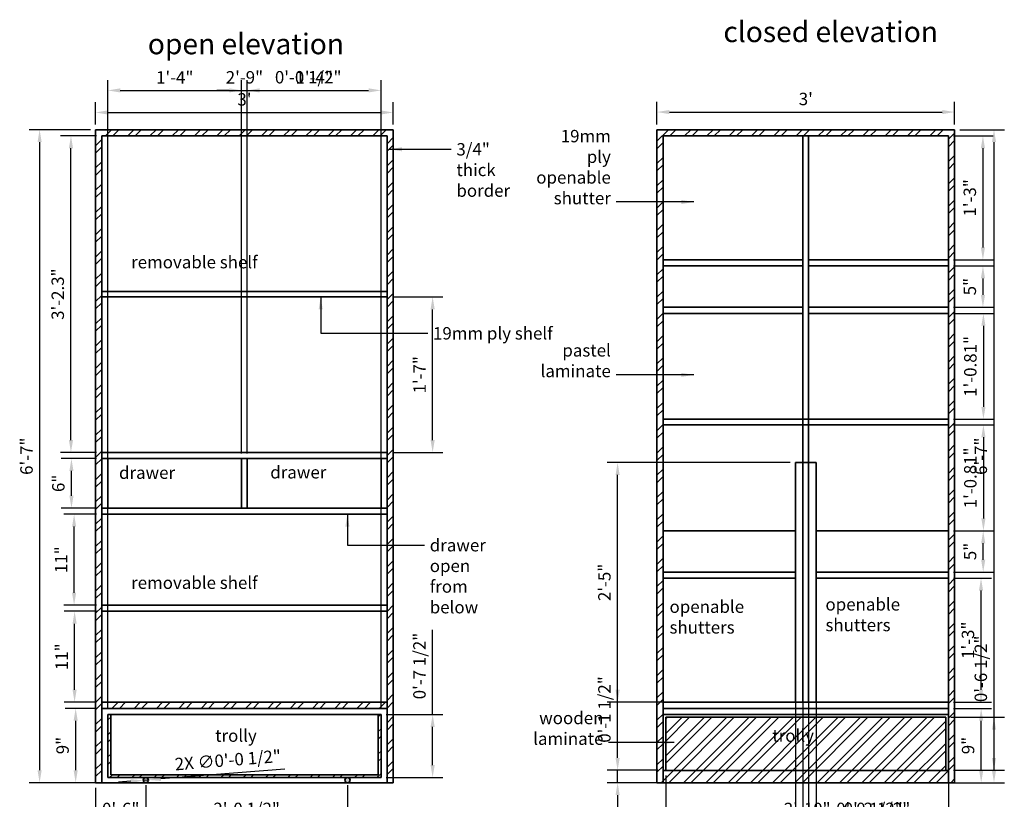
# Model space of a CAD drawing. Units: inches. Extents: x 1145 to 1264, y 2632 to 2775.
# Tile 2 of 2: x 1145 to 1264, y 2681 to 2775. Entities that reach past the tile are written whole.
import ezdxf

# ---------------------------------------------------------------- set-up
doc = ezdxf.new("R2010")
doc.units = ezdxf.units.IN
for name, color, linetype, lineweight in [('A-ANNO-DIMS', 2, 'Continuous', 18), ('A-ANNO-TEXT', 3, 'Continuous', 25), ('A-ELEV', 7, 'Continuous', 35), ('A-ELEV-PATT', 8, 'Continuous', 18)]:
    doc.layers.add(name, color=color, linetype=linetype, lineweight=lineweight)
doc.styles.get("Standard").update_dxf_attribs({"font": 'arial.ttf'})
doc.dimstyles.new('ISO-25', dxfattribs={"dimtxt": 1.5, "dimasz": 1.5, "dimexe": 1.25, "dimexo": 0.625, "dimtad": 1, "dimlunit": 3, "dimtxsty": 'Standard', "dimcen": 2.5, "dimadec": 0, "dimazin": 0, "dimtfac": 1, "dimtmove": 0, "dimatfit": 3, "dimfxl": 1, "dimarcsym": 0})

# ---------------------------------------------------------------- blocks, each defined once
blk = doc.blocks.new('*D3')
at = {"layer": 'A-ANNO-DIMS', "color": 0, "lineweight": -2, "transparency": 16777216}
for p, q in [((1154.04, 2691.52), (1150.26, 2691.52)), ((1151.51, 2684.02), (1151.51, 2690.02)), ((1154.04, 2682.52), (1150.26, 2682.52))]:
    blk.add_line(p, q, dxfattribs=at)
at = {"layer": 'A-ANNO-DIMS', "color": 0, "lineweight": 100, "transparency": 16777216}
for points in [[(1151.26, 2690.02), (1151.76, 2690.02), (1151.51, 2691.52)], [(1151.26, 2684.02), (1151.76, 2684.02), (1151.51, 2682.52)]]:
    blk.add_solid(points, dxfattribs=at)
at = {"layer": 'Defpoints', "color": 0, "lineweight": 100, "transparency": 16777216}
for p in [(1151.51, 2691.52), (1154.66, 2691.52), (1154.66, 2682.52)]:
    blk.add_point(p, dxfattribs=at)
at = {"layer": 'A-ANNO-DIMS', "color": 0, "transparency": 16777216, "insert": (1150.12, 2687.02), "char_height": 1.5, "attachment_point": 5, "rotation": 90}
blk.add_mtext('9"', dxfattribs=at)
blk = doc.blocks.new('*D4')
at = {"layer": 'A-ANNO-DIMS', "color": 0, "lineweight": -2, "transparency": 16777216}
for p, q in [((1154.04, 2703.26), (1150.13, 2703.26)), ((1151.38, 2693.76), (1151.38, 2701.76)), ((1154.04, 2692.26), (1150.13, 2692.26))]:
    blk.add_line(p, q, dxfattribs=at)
at = {"layer": 'A-ANNO-DIMS', "color": 0, "lineweight": 100, "transparency": 16777216}
for points in [[(1151.13, 2701.76), (1151.63, 2701.76), (1151.38, 2703.26)], [(1151.13, 2693.76), (1151.63, 2693.76), (1151.38, 2692.26)]]:
    blk.add_solid(points, dxfattribs=at)
at = {"layer": 'Defpoints', "color": 0, "lineweight": 100, "transparency": 16777216}
for p in [(1151.38, 2703.26), (1154.66, 2703.26), (1154.66, 2692.26)]:
    blk.add_point(p, dxfattribs=at)
at = {"layer": 'A-ANNO-DIMS', "color": 0, "transparency": 16777216, "insert": (1150.01, 2697.76), "char_height": 1.5, "attachment_point": 5, "rotation": 90}
blk.add_mtext('11"', dxfattribs=at)
blk = doc.blocks.new('*D5')
at = {"layer": 'A-ANNO-DIMS', "color": 0, "lineweight": -2, "transparency": 16777216}
for p, q in [((1154.04, 2715), (1150.07, 2715)), ((1151.32, 2705.5), (1151.32, 2713.5)), ((1154.04, 2704), (1150.07, 2704))]:
    blk.add_line(p, q, dxfattribs=at)
at = {"layer": 'A-ANNO-DIMS', "color": 0, "lineweight": 100, "transparency": 16777216}
for points in [[(1151.07, 2713.5), (1151.57, 2713.5), (1151.32, 2715)], [(1151.07, 2705.5), (1151.57, 2705.5), (1151.32, 2704)]]:
    blk.add_solid(points, dxfattribs=at)
at = {"layer": 'Defpoints', "color": 0, "lineweight": 100, "transparency": 16777216}
for p in [(1151.32, 2715), (1154.66, 2715), (1154.66, 2704)]:
    blk.add_point(p, dxfattribs=at)
at = {"layer": 'A-ANNO-DIMS', "color": 0, "transparency": 16777216, "insert": (1149.94, 2709.5), "char_height": 1.5, "attachment_point": 5, "rotation": 90}
blk.add_mtext('11"', dxfattribs=at)
blk = doc.blocks.new('*D6')
at = {"layer": 'A-ANNO-DIMS', "color": 0, "lineweight": -2, "transparency": 16777216}
for p, q in [((1154.04, 2721.74), (1149.75, 2721.74)), ((1151, 2717.24), (1151, 2720.24)), ((1154.04, 2715.74), (1149.75, 2715.74))]:
    blk.add_line(p, q, dxfattribs=at)
at = {"layer": 'A-ANNO-DIMS', "color": 0, "lineweight": 100, "transparency": 16777216}
for points in [[(1150.75, 2720.24), (1151.25, 2720.24), (1151, 2721.74)], [(1150.75, 2717.24), (1151.25, 2717.24), (1151, 2715.74)]]:
    blk.add_solid(points, dxfattribs=at)
at = {"layer": 'Defpoints', "color": 0, "lineweight": 100, "transparency": 16777216}
for p in [(1151, 2721.74), (1154.66, 2721.74), (1154.66, 2715.74)]:
    blk.add_point(p, dxfattribs=at)
at = {"layer": 'A-ANNO-DIMS', "color": 0, "transparency": 16777216, "insert": (1149.61, 2718.74), "char_height": 1.5, "attachment_point": 5, "rotation": 90}
blk.add_mtext('6"', dxfattribs=at)
blk = doc.blocks.new('*D7')
at = {"layer": 'A-ANNO-DIMS', "color": 0, "lineweight": -2, "transparency": 16777216}
for p, q in [((1154.04, 2760.78), (1149.69, 2760.78)), ((1150.94, 2723.98), (1150.94, 2759.28)), ((1154.04, 2722.48), (1149.69, 2722.48))]:
    blk.add_line(p, q, dxfattribs=at)
at = {"layer": 'A-ANNO-DIMS', "color": 0, "lineweight": 100, "transparency": 16777216}
for points in [[(1150.69, 2759.28), (1151.19, 2759.28), (1150.94, 2760.78)], [(1150.69, 2723.98), (1151.19, 2723.98), (1150.94, 2722.48)]]:
    blk.add_solid(points, dxfattribs=at)
at = {"layer": 'Defpoints', "color": 0, "lineweight": 100, "transparency": 16777216}
for p in [(1150.94, 2760.78), (1154.66, 2760.78), (1154.66, 2722.48)]:
    blk.add_point(p, dxfattribs=at)
at = {"layer": 'A-ANNO-DIMS', "color": 0, "transparency": 16777216, "insert": (1149.54, 2741.63), "char_height": 1.5, "attachment_point": 5, "rotation": 90}
blk.add_mtext('3\'-2.3"', dxfattribs=at)
blk = doc.blocks.new('*D8')
at = {"layer": 'A-ANNO-DIMS', "color": 0, "lineweight": -2, "transparency": 16777216}
for p, q in [((1153.92, 2762.14), (1153.92, 2764.86)), ((1189.92, 2762.14), (1189.92, 2764.86)), ((1155.42, 2763.61), (1188.42, 2763.61))]:
    blk.add_line(p, q, dxfattribs=at)
at = {"layer": 'A-ANNO-DIMS', "color": 0, "lineweight": 100, "transparency": 16777216}
for points in [[(1155.42, 2763.86), (1155.42, 2763.36), (1153.92, 2763.61)], [(1188.42, 2763.86), (1188.42, 2763.36), (1189.92, 2763.61)]]:
    blk.add_solid(points, dxfattribs=at)
at = {"layer": 'Defpoints', "color": 0, "lineweight": 100, "transparency": 16777216}
for p in [(1189.92, 2763.61), (1153.92, 2761.52), (1189.92, 2761.52)]:
    blk.add_point(p, dxfattribs=at)
at = {"layer": 'A-ANNO-DIMS', "color": 0, "transparency": 16777216, "insert": (1171.92, 2765), "char_height": 1.5, "attachment_point": 5}
blk.add_mtext("3'", dxfattribs=at)
blk = doc.blocks.new('*D9')
at = {"layer": 'A-ANNO-DIMS', "color": 0, "lineweight": -2, "transparency": 16777216}
for p, q in [((1153.3, 2761.52), (1145.9, 2761.52)), ((1147.15, 2760.02), (1147.15, 2684.02)), ((1153.3, 2682.52), (1145.9, 2682.52))]:
    blk.add_line(p, q, dxfattribs=at)
at = {"layer": 'A-ANNO-DIMS', "color": 0, "lineweight": 100, "transparency": 16777216}
for points in [[(1146.9, 2760.02), (1147.4, 2760.02), (1147.15, 2761.52)], [(1146.9, 2684.02), (1147.4, 2684.02), (1147.15, 2682.52)]]:
    blk.add_solid(points, dxfattribs=at)
at = {"layer": 'Defpoints', "color": 0, "lineweight": 100, "transparency": 16777216}
for p in [(1153.92, 2761.52), (1147.15, 2682.52), (1153.92, 2682.52)]:
    blk.add_point(p, dxfattribs=at)
at = {"layer": 'A-ANNO-DIMS', "color": 0, "transparency": 16777216, "insert": (1145.76, 2722.02), "char_height": 1.5, "attachment_point": 5, "rotation": 90}
blk.add_mtext('6\'-7"', dxfattribs=at)
blk = doc.blocks.new('*D10')
at = {"layer": 'A-ANNO-DIMS', "color": 0, "lineweight": -2, "transparency": 16777216}
for p, q in [((1221.81, 2762.14), (1221.81, 2764.91)), ((1257.81, 2762.14), (1257.81, 2764.91)), ((1223.31, 2763.66), (1256.31, 2763.66))]:
    blk.add_line(p, q, dxfattribs=at)
at = {"layer": 'A-ANNO-DIMS', "color": 0, "lineweight": 100, "transparency": 16777216}
for points in [[(1223.31, 2763.91), (1223.31, 2763.41), (1221.81, 2763.66)], [(1256.31, 2763.91), (1256.31, 2763.41), (1257.81, 2763.66)]]:
    blk.add_solid(points, dxfattribs=at)
at = {"layer": 'Defpoints', "color": 0, "lineweight": 100, "transparency": 16777216}
for p in [(1257.81, 2763.66), (1221.81, 2761.52), (1257.81, 2761.52)]:
    blk.add_point(p, dxfattribs=at)
at = {"layer": 'A-ANNO-DIMS', "color": 0, "transparency": 16777216, "insert": (1239.81, 2765.05), "char_height": 1.5, "attachment_point": 5}
blk.add_mtext("3'", dxfattribs=at)
blk = doc.blocks.new('*D11')
at = {"layer": 'A-ANNO-DIMS', "color": 0, "lineweight": -2, "transparency": 16777216}
for p, q in [((1257.69, 2691.52), (1262.27, 2691.52)), ((1261.02, 2684.02), (1261.02, 2690.02)), ((1257.69, 2682.52), (1262.27, 2682.52))]:
    blk.add_line(p, q, dxfattribs=at)
at = {"layer": 'A-ANNO-DIMS', "color": 0, "lineweight": 100, "transparency": 16777216}
for points in [[(1260.77, 2690.02), (1261.27, 2690.02), (1261.02, 2691.52)], [(1260.77, 2684.02), (1261.27, 2684.02), (1261.02, 2682.52)]]:
    blk.add_solid(points, dxfattribs=at)
at = {"layer": 'Defpoints', "color": 0, "lineweight": 100, "transparency": 16777216}
for p in [(1257.07, 2691.52), (1261.02, 2691.52), (1257.07, 2682.52)]:
    blk.add_point(p, dxfattribs=at)
at = {"layer": 'A-ANNO-DIMS', "color": 0, "transparency": 16777216, "insert": (1259.63, 2687.02), "char_height": 1.5, "attachment_point": 5, "rotation": 90}
blk.add_mtext('9"', dxfattribs=at)
blk = doc.blocks.new('*D12')
at = {"layer": 'A-ANNO-DIMS', "color": 0, "lineweight": -2, "transparency": 16777216}
for p, q in [((1257.69, 2707.26), (1262.25, 2707.26)), ((1261, 2693.76), (1261, 2705.76)), ((1257.69, 2692.26), (1262.25, 2692.26))]:
    blk.add_line(p, q, dxfattribs=at)
at = {"layer": 'A-ANNO-DIMS', "color": 0, "lineweight": 100, "transparency": 16777216}
for points in [[(1260.75, 2705.76), (1261.25, 2705.76), (1261, 2707.26)], [(1260.75, 2693.76), (1261.25, 2693.76), (1261, 2692.26)]]:
    blk.add_solid(points, dxfattribs=at)
at = {"layer": 'Defpoints', "color": 0, "lineweight": 100, "transparency": 16777216}
for p in [(1257.07, 2707.26), (1261, 2707.26), (1257.07, 2692.26)]:
    blk.add_point(p, dxfattribs=at)
at = {"layer": 'A-ANNO-DIMS', "color": 0, "transparency": 16777216, "insert": (1259.61, 2699.76), "char_height": 1.5, "attachment_point": 5, "rotation": 90}
blk.add_mtext('1\'-3"', dxfattribs=at)
blk = doc.blocks.new('*D13')
at = {"layer": 'A-ANNO-DIMS', "color": 0, "lineweight": -2, "transparency": 16777216}
for p, q in [((1257.69, 2713), (1262.51, 2713)), ((1261.26, 2709.5), (1261.26, 2711.5)), ((1257.69, 2708), (1262.51, 2708))]:
    blk.add_line(p, q, dxfattribs=at)
at = {"layer": 'A-ANNO-DIMS', "color": 0, "lineweight": 100, "transparency": 16777216}
for points in [[(1261.01, 2711.5), (1261.51, 2711.5), (1261.26, 2713)], [(1261.01, 2709.5), (1261.51, 2709.5), (1261.26, 2708)]]:
    blk.add_solid(points, dxfattribs=at)
at = {"layer": 'Defpoints', "color": 0, "lineweight": 100, "transparency": 16777216}
for p in [(1257.07, 2713), (1261.26, 2713), (1257.07, 2708)]:
    blk.add_point(p, dxfattribs=at)
at = {"layer": 'A-ANNO-DIMS', "color": 0, "transparency": 16777216, "insert": (1259.87, 2710.5), "char_height": 1.5, "attachment_point": 5, "rotation": 90}
blk.add_mtext('5"', dxfattribs=at)
blk = doc.blocks.new('*D14')
at = {"layer": 'A-ANNO-DIMS', "color": 0, "lineweight": -2, "transparency": 16777216}
for p, q in [((1257.69, 2760.78), (1262.48, 2760.78)), ((1261.23, 2759.28), (1261.23, 2747.28)), ((1257.69, 2745.78), (1262.48, 2745.78))]:
    blk.add_line(p, q, dxfattribs=at)
at = {"layer": 'A-ANNO-DIMS', "color": 0, "lineweight": 100, "transparency": 16777216}
for points in [[(1260.98, 2759.28), (1261.48, 2759.28), (1261.23, 2760.78)], [(1260.98, 2747.28), (1261.48, 2747.28), (1261.23, 2745.78)]]:
    blk.add_solid(points, dxfattribs=at)
at = {"layer": 'Defpoints', "color": 0, "lineweight": 100, "transparency": 16777216}
for p in [(1257.07, 2760.78), (1257.07, 2745.78), (1261.23, 2745.78)]:
    blk.add_point(p, dxfattribs=at)
at = {"layer": 'A-ANNO-DIMS', "color": 0, "transparency": 16777216, "insert": (1259.84, 2753.28), "char_height": 1.5, "attachment_point": 5, "rotation": 90}
blk.add_mtext('1\'-3"', dxfattribs=at)
blk = doc.blocks.new('*D15')
at = {"layer": 'A-ANNO-DIMS', "color": 0, "lineweight": -2, "transparency": 16777216}
for p, q in [((1257.69, 2745.04), (1262.48, 2745.04)), ((1261.23, 2743.54), (1261.23, 2741.54)), ((1257.69, 2740.04), (1262.48, 2740.04))]:
    blk.add_line(p, q, dxfattribs=at)
at = {"layer": 'A-ANNO-DIMS', "color": 0, "lineweight": 100, "transparency": 16777216}
for points in [[(1260.98, 2743.54), (1261.48, 2743.54), (1261.23, 2745.04)], [(1260.98, 2741.54), (1261.48, 2741.54), (1261.23, 2740.04)]]:
    blk.add_solid(points, dxfattribs=at)
at = {"layer": 'Defpoints', "color": 0, "lineweight": 100, "transparency": 16777216}
for p in [(1257.07, 2745.04), (1257.07, 2740.04), (1261.23, 2740.04)]:
    blk.add_point(p, dxfattribs=at)
at = {"layer": 'A-ANNO-DIMS', "color": 0, "transparency": 16777216, "insert": (1259.84, 2742.54), "char_height": 1.5, "attachment_point": 5, "rotation": 90}
blk.add_mtext('5"', dxfattribs=at)
blk = doc.blocks.new('*D16')
at = {"layer": 'A-ANNO-DIMS', "color": 0, "lineweight": -2, "transparency": 16777216}
for p, q in [((1257.69, 2739.3), (1262.54, 2739.3)), ((1261.29, 2737.8), (1261.29, 2727.99)), ((1257.69, 2726.49), (1262.54, 2726.49))]:
    blk.add_line(p, q, dxfattribs=at)
at = {"layer": 'A-ANNO-DIMS', "color": 0, "lineweight": 100, "transparency": 16777216}
for points in [[(1261.04, 2737.8), (1261.54, 2737.8), (1261.29, 2739.3)], [(1261.04, 2727.99), (1261.54, 2727.99), (1261.29, 2726.49)]]:
    blk.add_solid(points, dxfattribs=at)
at = {"layer": 'Defpoints', "color": 0, "lineweight": 100, "transparency": 16777216}
for p in [(1257.07, 2739.3), (1257.07, 2726.49), (1261.29, 2726.49)]:
    blk.add_point(p, dxfattribs=at)
at = {"layer": 'A-ANNO-DIMS', "color": 0, "transparency": 16777216, "insert": (1259.9, 2732.89), "char_height": 1.5, "attachment_point": 5, "rotation": 90}
blk.add_mtext('1\'-0.81"', dxfattribs=at)
blk = doc.blocks.new('*D17')
at = {"layer": 'A-ANNO-DIMS', "color": 0, "lineweight": -2, "transparency": 16777216}
for p, q in [((1257.69, 2725.81), (1262.54, 2725.81)), ((1261.29, 2724.31), (1261.29, 2714.5)), ((1257.69, 2713), (1262.54, 2713))]:
    blk.add_line(p, q, dxfattribs=at)
at = {"layer": 'A-ANNO-DIMS', "color": 0, "lineweight": 100, "transparency": 16777216}
for points in [[(1261.04, 2724.31), (1261.54, 2724.31), (1261.29, 2725.81)], [(1261.04, 2714.5), (1261.54, 2714.5), (1261.29, 2713)]]:
    blk.add_solid(points, dxfattribs=at)
at = {"layer": 'Defpoints', "color": 0, "lineweight": 100, "transparency": 16777216}
for p in [(1257.07, 2725.81), (1257.07, 2713), (1261.29, 2713)]:
    blk.add_point(p, dxfattribs=at)
at = {"layer": 'A-ANNO-DIMS', "color": 0, "transparency": 16777216, "insert": (1259.9, 2719.4), "char_height": 1.5, "attachment_point": 5, "rotation": 90}
blk.add_mtext('1\'-0.81"', dxfattribs=at)
blk = doc.blocks.new('*D18')
at = {"layer": 'A-ANNO-DIMS', "color": 0, "lineweight": -2, "transparency": 16777216}
for p, q in [((1189.81, 2741.29), (1195.93, 2741.29)), ((1194.68, 2723.98), (1194.68, 2739.79)), ((1189.81, 2722.48), (1195.93, 2722.48))]:
    blk.add_line(p, q, dxfattribs=at)
at = {"layer": 'A-ANNO-DIMS', "color": 0, "lineweight": 100, "transparency": 16777216}
for points in [[(1194.43, 2739.79), (1194.93, 2739.79), (1194.68, 2741.29)], [(1194.43, 2723.98), (1194.93, 2723.98), (1194.68, 2722.48)]]:
    blk.add_solid(points, dxfattribs=at)
at = {"layer": 'Defpoints', "color": 0, "lineweight": 100, "transparency": 16777216}
for p in [(1189.18, 2741.29), (1194.68, 2741.29), (1189.18, 2722.48)]:
    blk.add_point(p, dxfattribs=at)
at = {"layer": 'A-ANNO-DIMS', "color": 0, "transparency": 16777216, "insert": (1193.3, 2731.88), "char_height": 1.5, "attachment_point": 5, "rotation": 90}
blk.add_mtext('1\'-7"', dxfattribs=at)
blk = doc.blocks.new('*D19')
at = {"layer": 'A-ANNO-DIMS', "color": 0, "lineweight": -2, "transparency": 16777216}
for p, q in [((1155.4, 2691.4), (1155.4, 2767.53)), ((1188.44, 2691.4), (1188.44, 2767.53)), ((1156.9, 2766.28), (1186.94, 2766.28))]:
    blk.add_line(p, q, dxfattribs=at)
at = {"layer": 'A-ANNO-DIMS', "color": 0, "lineweight": 100, "transparency": 16777216}
for points in [[(1156.9, 2766.53), (1156.9, 2766.03), (1155.4, 2766.28)], [(1186.94, 2766.53), (1186.94, 2766.03), (1188.44, 2766.28)]]:
    blk.add_solid(points, dxfattribs=at)
at = {"layer": 'Defpoints', "color": 0, "lineweight": 100, "transparency": 16777216}
for p in [(1188.44, 2766.28), (1155.4, 2690.78), (1188.44, 2690.78)]:
    blk.add_point(p, dxfattribs=at)
at = {"layer": 'A-ANNO-DIMS', "color": 0, "transparency": 16777216, "insert": (1171.92, 2767.67), "char_height": 1.5, "attachment_point": 5}
blk.add_mtext('2\'-9"', dxfattribs=at)
blk = doc.blocks.new('*D20')
at = {"layer": 'A-ANNO-DIMS', "color": 0, "lineweight": -2, "transparency": 16777216}
for p, q in [((1194.68, 2690.78), (1194.68, 2701.01)), ((1189.07, 2690.78), (1195.93, 2690.78)), ((1194.68, 2684.65), (1194.68, 2689.28)), ((1189.07, 2683.15), (1195.93, 2683.15))]:
    blk.add_line(p, q, dxfattribs=at)
at = {"layer": 'A-ANNO-DIMS', "color": 0, "lineweight": 100, "transparency": 16777216}
for points in [[(1194.43, 2689.28), (1194.93, 2689.28), (1194.68, 2690.78)], [(1194.43, 2684.65), (1194.93, 2684.65), (1194.68, 2683.15)]]:
    blk.add_solid(points, dxfattribs=at)
at = {"layer": 'Defpoints', "color": 0, "lineweight": 100, "transparency": 16777216}
for p in [(1188.44, 2690.78), (1194.68, 2690.78), (1188.44, 2683.15)]:
    blk.add_point(p, dxfattribs=at)
at = {"layer": 'A-ANNO-DIMS', "color": 0, "transparency": 16777216, "insert": (1193.28, 2696.64), "char_height": 1.5, "attachment_point": 5, "rotation": 90}
blk.add_mtext('0\'-7 1/2"', dxfattribs=at)
blk = doc.blocks.new('*D21')
at = {"layer": 'A-ANNO-DIMS', "color": 0, "lineweight": -2, "transparency": 16777216}
for p, q in [((1153.92, 2681.89), (1153.92, 2676.51)), ((1159.99, 2682.21), (1159.99, 2676.51)), ((1155.42, 2677.76), (1158.49, 2677.76))]:
    blk.add_line(p, q, dxfattribs=at)
at = {"layer": 'A-ANNO-DIMS', "color": 0, "lineweight": 100, "transparency": 16777216}
for points in [[(1155.42, 2678.01), (1155.42, 2677.51), (1153.92, 2677.76)], [(1158.49, 2678.01), (1158.49, 2677.51), (1159.99, 2677.76)]]:
    blk.add_solid(points, dxfattribs=at)
at = {"layer": 'Defpoints', "color": 0, "lineweight": 100, "transparency": 16777216}
for p in [(1159.99, 2682.84), (1153.92, 2682.52), (1159.99, 2677.76)]:
    blk.add_point(p, dxfattribs=at)
at = {"layer": 'A-ANNO-DIMS', "color": 0, "transparency": 16777216, "insert": (1156.96, 2679.15), "char_height": 1.5, "attachment_point": 5}
blk.add_mtext('0\'-6"', dxfattribs=at)
blk = doc.blocks.new('*D22')
at = {"layer": 'A-ANNO-DIMS', "color": 0, "lineweight": -2, "transparency": 16777216}
for p, q in [((1159.99, 2682.21), (1159.99, 2676.51)), ((1184.39, 2682.21), (1184.39, 2676.51)), ((1161.49, 2677.76), (1182.89, 2677.76))]:
    blk.add_line(p, q, dxfattribs=at)
at = {"layer": 'A-ANNO-DIMS', "color": 0, "lineweight": 100, "transparency": 16777216}
for points in [[(1161.49, 2678.01), (1161.49, 2677.51), (1159.99, 2677.76)], [(1182.89, 2678.01), (1182.89, 2677.51), (1184.39, 2677.76)]]:
    blk.add_solid(points, dxfattribs=at)
at = {"layer": 'Defpoints', "color": 0, "lineweight": 100, "transparency": 16777216}
for p in [(1159.99, 2682.84), (1184.39, 2682.84), (1184.39, 2677.76)]:
    blk.add_point(p, dxfattribs=at)
at = {"layer": 'A-ANNO-DIMS', "color": 0, "transparency": 16777216, "insert": (1172.19, 2679.16), "char_height": 1.5, "attachment_point": 5}
blk.add_mtext('2\'-0 1/2"', dxfattribs=at)
blk = doc.blocks.new('*D23')
at = {"layer": 'A-ANNO-DIMS', "color": 0, "lineweight": -2, "transparency": 16777216}
for p, q in [((1155.4, 2722.36), (1155.4, 2767.53)), ((1171.58, 2722.36), (1171.58, 2767.53)), ((1156.9, 2766.28), (1170.08, 2766.28))]:
    blk.add_line(p, q, dxfattribs=at)
at = {"layer": 'A-ANNO-DIMS', "color": 0, "lineweight": 100, "transparency": 16777216}
for points in [[(1156.9, 2766.53), (1156.9, 2766.03), (1155.4, 2766.28)], [(1170.08, 2766.53), (1170.08, 2766.03), (1171.58, 2766.28)]]:
    blk.add_solid(points, dxfattribs=at)
at = {"layer": 'Defpoints', "color": 0, "lineweight": 100, "transparency": 16777216}
for p in [(1171.58, 2766.28), (1155.4, 2721.74), (1171.58, 2721.74)]:
    blk.add_point(p, dxfattribs=at)
at = {"layer": 'A-ANNO-DIMS', "color": 0, "transparency": 16777216, "insert": (1163.49, 2767.66), "char_height": 1.5, "attachment_point": 5}
blk.add_mtext('1\'-4"', dxfattribs=at)
blk = doc.blocks.new('*D24')
at = {"layer": 'A-ANNO-DIMS', "color": 0, "lineweight": -2, "transparency": 16777216}
for p, q in [((1171.58, 2722.36), (1171.58, 2767.53)), ((1172.26, 2722.36), (1172.26, 2767.53)), ((1170.08, 2766.28), (1168.58, 2766.28)), ((1171.58, 2766.28), (1172.26, 2766.28)), ((1173.76, 2766.28), (1184, 2766.28))]:
    blk.add_line(p, q, dxfattribs=at)
at = {"layer": 'A-ANNO-DIMS', "color": 0, "lineweight": 100, "transparency": 16777216}
for points in [[(1170.08, 2766.53), (1170.08, 2766.03), (1171.58, 2766.28)], [(1173.76, 2766.53), (1173.76, 2766.03), (1172.26, 2766.28)]]:
    blk.add_solid(points, dxfattribs=at)
at = {"layer": 'Defpoints', "color": 0, "lineweight": 100, "transparency": 16777216}
for p in [(1172.26, 2766.28), (1171.58, 2721.74), (1172.26, 2721.74)]:
    blk.add_point(p, dxfattribs=at)
at = {"layer": 'A-ANNO-DIMS', "color": 0, "transparency": 16777216, "insert": (1179.63, 2767.68), "char_height": 1.5, "attachment_point": 5}
blk.add_mtext('0\'-0 1/2"', dxfattribs=at)
blk = doc.blocks.new('*D25')
at = {"layer": 'A-ANNO-DIMS', "color": 0, "lineweight": -2, "transparency": 16777216}
for p, q in [((1172.26, 2722.36), (1172.26, 2767.53)), ((1188.44, 2722.36), (1188.44, 2767.53)), ((1173.76, 2766.28), (1186.94, 2766.28))]:
    blk.add_line(p, q, dxfattribs=at)
at = {"layer": 'A-ANNO-DIMS', "color": 0, "lineweight": 100, "transparency": 16777216}
for points in [[(1173.76, 2766.53), (1173.76, 2766.03), (1172.26, 2766.28)], [(1186.94, 2766.53), (1186.94, 2766.03), (1188.44, 2766.28)]]:
    blk.add_solid(points, dxfattribs=at)
at = {"layer": 'Defpoints', "color": 0, "lineweight": 100, "transparency": 16777216}
for p in [(1188.44, 2766.28), (1172.26, 2721.74), (1188.44, 2721.74)]:
    blk.add_point(p, dxfattribs=at)
at = {"layer": 'A-ANNO-DIMS', "color": 0, "transparency": 16777216, "insert": (1180.35, 2767.66), "char_height": 1.5, "attachment_point": 5}
blk.add_mtext('1\'-4"', dxfattribs=at)
blk = doc.blocks.new('*D26')
at = {"layer": 'A-ANNO-DIMS', "color": 0, "lineweight": -2, "transparency": 16777216}
for p, q in [((1238.56, 2720.63), (1238.56, 2676.51)), ((1241.06, 2720.63), (1241.06, 2676.51)), ((1237.06, 2677.76), (1235.56, 2677.76)), ((1238.56, 2677.76), (1241.06, 2677.76)), ((1242.56, 2677.76), (1252.79, 2677.76))]:
    blk.add_line(p, q, dxfattribs=at)
at = {"layer": 'A-ANNO-DIMS', "color": 0, "lineweight": 100, "transparency": 16777216}
for points in [[(1237.06, 2678.01), (1237.06, 2677.51), (1238.56, 2677.76)], [(1242.56, 2678.01), (1242.56, 2677.51), (1241.06, 2677.76)]]:
    blk.add_solid(points, dxfattribs=at)
at = {"layer": 'Defpoints', "color": 0, "lineweight": 100, "transparency": 16777216}
for p in [(1238.56, 2721.26), (1241.06, 2721.26), (1241.06, 2677.76)]:
    blk.add_point(p, dxfattribs=at)
at = {"layer": 'A-ANNO-DIMS', "color": 0, "transparency": 16777216, "insert": (1248.42, 2679.16), "char_height": 1.5, "attachment_point": 5}
blk.add_mtext('0\'-2 1/2"', dxfattribs=at)
blk = doc.blocks.new('*D27')
at = {"layer": 'A-ANNO-DIMS', "color": 0, "lineweight": -2, "transparency": 16777216}
for p, q in [((1237.93, 2721.26), (1215.8, 2721.26)), ((1217.05, 2693.76), (1217.05, 2719.76)), ((1237.93, 2692.26), (1215.8, 2692.26))]:
    blk.add_line(p, q, dxfattribs=at)
at = {"layer": 'A-ANNO-DIMS', "color": 0, "lineweight": 100, "transparency": 16777216}
for points in [[(1216.8, 2719.76), (1217.3, 2719.76), (1217.05, 2721.26)], [(1216.8, 2693.76), (1217.3, 2693.76), (1217.05, 2692.26)]]:
    blk.add_solid(points, dxfattribs=at)
at = {"layer": 'Defpoints', "color": 0, "lineweight": 100, "transparency": 16777216}
for p in [(1217.05, 2721.26), (1238.56, 2721.26), (1238.56, 2692.26)]:
    blk.add_point(p, dxfattribs=at)
at = {"layer": 'A-ANNO-DIMS', "color": 0, "transparency": 16777216, "insert": (1215.65, 2706.76), "char_height": 1.5, "attachment_point": 5, "rotation": 90}
blk.add_mtext('2\'-5"', dxfattribs=at)
blk = doc.blocks.new('*D28')
at = {"layer": 'A-ANNO-DIMS', "color": 0, "lineweight": -2, "transparency": 16777216}
for p, q in [((1239.47, 2760.15), (1239.47, 2676.51)), ((1240.15, 2760.15), (1240.15, 2676.51)), ((1237.97, 2677.76), (1236.47, 2677.76)), ((1239.47, 2677.76), (1240.15, 2677.76)), ((1241.65, 2677.76), (1251.88, 2677.76))]:
    blk.add_line(p, q, dxfattribs=at)
at = {"layer": 'A-ANNO-DIMS', "color": 0, "lineweight": 100, "transparency": 16777216}
for points in [[(1237.97, 2678.01), (1237.97, 2677.51), (1239.47, 2677.76)], [(1241.65, 2678.01), (1241.65, 2677.51), (1240.15, 2677.76)]]:
    blk.add_solid(points, dxfattribs=at)
at = {"layer": 'Defpoints', "color": 0, "lineweight": 100, "transparency": 16777216}
for p in [(1239.47, 2760.78), (1240.15, 2760.78), (1240.15, 2677.76)]:
    blk.add_point(p, dxfattribs=at)
at = {"layer": 'A-ANNO-DIMS', "color": 0, "transparency": 16777216, "insert": (1247.51, 2679.16), "char_height": 1.5, "attachment_point": 5}
blk.add_mtext('0\'-0 1/2"', dxfattribs=at)
blk = doc.blocks.new('*D29')
at = {"layer": 'A-ANNO-DIMS', "color": 0, "lineweight": -2, "transparency": 16777216}
for p, q in [((1222.89, 2683.39), (1222.89, 2676.51)), ((1257.07, 2683.39), (1257.07, 2676.51)), ((1224.39, 2677.76), (1255.57, 2677.76))]:
    blk.add_line(p, q, dxfattribs=at)
at = {"layer": 'A-ANNO-DIMS', "color": 0, "lineweight": 100, "transparency": 16777216}
for points in [[(1224.39, 2678.01), (1224.39, 2677.51), (1222.89, 2677.76)], [(1255.57, 2678.01), (1255.57, 2677.51), (1257.07, 2677.76)]]:
    blk.add_solid(points, dxfattribs=at)
at = {"layer": 'Defpoints', "color": 0, "lineweight": 100, "transparency": 16777216}
for p in [(1222.89, 2684.02), (1257.07, 2684.02), (1257.07, 2677.76)]:
    blk.add_point(p, dxfattribs=at)
at = {"layer": 'A-ANNO-DIMS', "color": 0, "transparency": 16777216, "insert": (1239.98, 2679.15), "char_height": 1.5, "attachment_point": 5}
blk.add_mtext('2\'-10"', dxfattribs=at)
blk = doc.blocks.new('*D30')
at = {"layer": 'A-ANNO-DIMS', "color": 0, "lineweight": -2, "transparency": 16777216}
for p, q in [((1262.57, 2690.44), (1262.57, 2700.67)), ((1257.35, 2690.44), (1263.82, 2690.44)), ((1262.57, 2685.52), (1262.57, 2688.94)), ((1257.69, 2684.02), (1263.82, 2684.02))]:
    blk.add_line(p, q, dxfattribs=at)
at = {"layer": 'A-ANNO-DIMS', "color": 0, "lineweight": 100, "transparency": 16777216}
for points in [[(1262.32, 2688.94), (1262.82, 2688.94), (1262.57, 2690.44)], [(1262.32, 2685.52), (1262.82, 2685.52), (1262.57, 2684.02)]]:
    blk.add_solid(points, dxfattribs=at)
at = {"layer": 'Defpoints', "color": 0, "lineweight": 100, "transparency": 16777216}
for p in [(1256.73, 2690.44), (1262.57, 2690.44), (1257.07, 2684.02)]:
    blk.add_point(p, dxfattribs=at)
at = {"layer": 'A-ANNO-DIMS', "color": 0, "transparency": 16777216, "insert": (1261.17, 2696.3), "char_height": 1.5, "attachment_point": 5, "rotation": 90}
blk.add_mtext('0\'-6 1/2"', dxfattribs=at)
blk = doc.blocks.new('*D31')
at = {"layer": 'A-ANNO-DIMS', "color": 0, "lineweight": -2, "transparency": 16777216}
for p, q in [((1217.05, 2685.52), (1217.05, 2695.75)), ((1221.92, 2684.02), (1215.8, 2684.02)), ((1217.05, 2682.52), (1217.05, 2684.02)), ((1221.92, 2682.52), (1215.8, 2682.52)), ((1217.05, 2681.02), (1217.05, 2679.52))]:
    blk.add_line(p, q, dxfattribs=at)
at = {"layer": 'A-ANNO-DIMS', "color": 0, "lineweight": 100, "transparency": 16777216}
for points in [[(1216.8, 2685.52), (1217.3, 2685.52), (1217.05, 2684.02)], [(1216.8, 2681.02), (1217.3, 2681.02), (1217.05, 2682.52)]]:
    blk.add_solid(points, dxfattribs=at)
at = {"layer": 'Defpoints', "color": 0, "lineweight": 100, "transparency": 16777216}
for p in [(1217.05, 2684.02), (1222.55, 2684.02), (1222.55, 2682.52)]:
    blk.add_point(p, dxfattribs=at)
at = {"layer": 'A-ANNO-DIMS', "color": 0, "transparency": 16777216, "insert": (1215.65, 2691.38), "char_height": 1.5, "attachment_point": 5, "rotation": 90}
blk.add_mtext('0\'-1 1/2"', dxfattribs=at)
blk = doc.blocks.new('*D32')
at = {"layer": 'A-ANNO-DIMS', "color": 0, "lineweight": -2, "transparency": 16777216}
for p, q in [((1258.43, 2761.52), (1263.82, 2761.52)), ((1262.57, 2684.02), (1262.57, 2760.02)), ((1258.43, 2682.52), (1263.82, 2682.52))]:
    blk.add_line(p, q, dxfattribs=at)
at = {"layer": 'A-ANNO-DIMS', "color": 0, "lineweight": 100, "transparency": 16777216}
for points in [[(1262.32, 2760.02), (1262.82, 2760.02), (1262.57, 2761.52)], [(1262.32, 2684.02), (1262.82, 2684.02), (1262.57, 2682.52)]]:
    blk.add_solid(points, dxfattribs=at)
at = {"layer": 'Defpoints', "color": 0, "lineweight": 100, "transparency": 16777216}
for p in [(1257.81, 2761.52), (1262.57, 2761.52), (1257.81, 2682.52)]:
    blk.add_point(p, dxfattribs=at)
at = {"layer": 'A-ANNO-DIMS', "color": 0, "transparency": 16777216, "insert": (1261.17, 2722.02), "char_height": 1.5, "attachment_point": 5, "rotation": 90}
blk.add_mtext('6\'-7"', dxfattribs=at)
blk = doc.blocks.new('*D38')
at = {"layer": 'A-ANNO-DIMS', "color": 0, "lineweight": -2, "transparency": 16777216}
for p, q in [((1176.79, 2684.17), (1161.8, 2682.98)), ((1159.67, 2682.81), (1160.31, 2682.86)), ((1158.18, 2682.69), (1156.68, 2682.57))]:
    blk.add_line(p, q, dxfattribs=at)
at = {"layer": 'A-ANNO-DIMS', "color": 0, "lineweight": 100, "transparency": 16777216}
for points in [[(1158.16, 2682.94), (1158.2, 2682.44), (1159.67, 2682.81)], [(1161.78, 2683.23), (1161.82, 2682.73), (1160.31, 2682.86)]]:
    blk.add_solid(points, dxfattribs=at)
at = {"layer": 'Defpoints', "color": 0, "lineweight": 100, "transparency": 16777216}
for p in [(1159.67, 2682.81), (1160.31, 2682.86)]:
    blk.add_point(p, dxfattribs=at)
at = {"layer": 'A-ANNO-DIMS', "color": 0, "transparency": 16777216, "insert": (1169.93, 2685.07), "char_height": 1.5, "attachment_point": 5, "rotation": 4.5545}
blk.add_mtext('2X ∅0\'-0 1/2"', dxfattribs=at)

msp = doc.modelspace()

# ---------------------------------------------------------------- hatches: boundary and pattern name
at = {"layer": 'A-ELEV-PATT'}
h = msp.add_hatch(dxfattribs=at)
h.set_pattern_fill('ANSI32', color=256, scale=0.2)
h.paths.add_polyline_path([(1189.923, 2761.518), (1153.923, 2761.518), (1153.923, 2682.518), (1154.663, 2682.518), (1154.663, 2760.778), (1189.183, 2760.778), (1189.183, 2682.518), (1189.923, 2682.518)])
h.paths.add_polyline_path([(1188.443, 2690.778), (1188.103, 2690.778), (1188.103, 2683.494), (1155.743, 2683.494), (1155.743, 2690.778), (1155.403, 2690.778), (1155.403, 2683.154), (1188.443, 2683.154)], flags=17)
h.paths.add_polyline_path([(1189.183, 2692.258), (1154.663, 2692.258), (1154.663, 2691.518), (1189.183, 2691.518)], flags=17)
h = msp.add_hatch(dxfattribs=at)
h.set_pattern_fill('ANSI32', color=256, scale=0.2)
h.paths.add_polyline_path([(1256.726, 2690.438), (1222.886, 2690.438), (1222.886, 2684.018), (1256.726, 2684.018)], flags=17)
h.paths.add_polyline_path([(1257.066, 2684.018), (1222.546, 2684.018), (1222.546, 2682.518), (1257.066, 2682.518)], flags=17)
h.paths.add_polyline_path([(1222.546, 2760.778), (1257.066, 2760.778), (1257.066, 2682.518), (1257.806, 2682.518), (1257.806, 2761.518), (1221.806, 2761.518), (1221.806, 2682.518), (1222.546, 2682.518), (1222.546, 2684.018)])
h = msp.add_hatch(color=256, dxfattribs=at)
h.dxf.hatch_style = 1
h.paths.add_polyline_path([(1184.705, 2682.836, 1), (1184.07, 2682.836, 1)])
h.paths.add_polyline_path([(1159.673, 2682.836, 1), (1160.308, 2682.836, 1)])

# ---------------------------------------------------------------- linework, layer by layer
at = {"layer": 'A-ELEV'}
for p, q in [((1189.923, 2761.518), (1153.923, 2761.518)), ((1153.923, 2761.518), (1153.923, 2682.518)), ((1189.923, 2682.518), (1189.923, 2761.518)), ((1221.806, 2761.518), (1257.806, 2761.518)), ((1221.806, 2682.518), (1221.806, 2761.518)), ((1257.806, 2761.518), (1257.806, 2682.518)), ((1154.663, 2760.778), (1154.663, 2682.518)), ((1189.183, 2760.778), (1154.663, 2760.778)), ((1189.183, 2682.518), (1189.183, 2760.778)), ((1222.546, 2760.778), (1257.066, 2760.778)), ((1222.546, 2682.518), (1222.546, 2760.778)), ((1239.466, 2760.778), (1239.466, 2692.258)), ((1240.146, 2760.778), (1240.146, 2692.258)), ((1257.066, 2760.778), (1257.066, 2682.518)), ((1222.546, 2745.778), (1239.466, 2745.778)), ((1222.546, 2745.038), (1239.466, 2745.038)), ((1240.146, 2745.778), (1257.066, 2745.778)), ((1240.146, 2745.038), (1257.066, 2745.038)), ((1154.663, 2741.968), (1189.183, 2741.968)), ((1154.663, 2741.288), (1189.183, 2741.288)), ((1222.546, 2740.038), (1239.466, 2740.038)), ((1240.146, 2740.038), (1257.066, 2740.038)), ((1222.546, 2739.298), (1239.466, 2739.298)), ((1240.146, 2739.298), (1257.066, 2739.298)), ((1257.066, 2739.298), (1257.066, 2712.998)), ((1257.066, 2726.488), (1222.546, 2726.488)), ((1257.066, 2725.808), (1222.546, 2725.808)), ((1154.663, 2722.478), (1189.183, 2722.478)), ((1154.663, 2721.738), (1189.183, 2721.738)), ((1155.403, 2721.738), (1155.403, 2715.738)), ((1155.403, 2721.738), (1188.443, 2721.738)), ((1171.583, 2721.738), (1171.583, 2715.738)), ((1172.263, 2721.738), (1172.263, 2715.738)), ((1188.443, 2715.738), (1188.443, 2721.738)), ((1241.056, 2721.258), (1238.556, 2721.258)), ((1238.556, 2721.258), (1238.556, 2692.258)), ((1241.056, 2692.258), (1241.056, 2721.258)), ((1154.663, 2715.738), (1189.183, 2715.738)), ((1154.663, 2714.998), (1189.183, 2714.998)), ((1238.556, 2712.998), (1222.546, 2712.998)), ((1257.066, 2712.998), (1241.056, 2712.998)), ((1238.556, 2707.998), (1222.546, 2707.998)), ((1257.066, 2707.998), (1241.056, 2707.998)), ((1238.556, 2707.258), (1222.546, 2707.258)), ((1257.066, 2707.258), (1241.056, 2707.258)), ((1154.663, 2703.998), (1189.183, 2703.998)), ((1154.663, 2703.258), (1189.183, 2703.258)), ((1154.663, 2692.258), (1189.183, 2692.258)), ((1154.663, 2691.518), (1189.183, 2691.518)), ((1257.066, 2692.258), (1222.546, 2692.258)), ((1257.066, 2691.518), (1222.546, 2691.518)), ((1238.556, 2692.258), (1241.056, 2692.258)), ((1155.403, 2690.778), (1188.443, 2690.778)), ((1155.403, 2690.778), (1155.403, 2683.154)), ((1155.743, 2690.778), (1155.743, 2683.494)), ((1188.103, 2683.494), (1188.103, 2690.778)), ((1188.443, 2683.154), (1188.443, 2690.778)), ((1257.066, 2690.778), (1222.546, 2690.778)), ((1256.726, 2690.438), (1222.886, 2690.438)), ((1222.886, 2684.018), (1222.886, 2690.438)), ((1256.726, 2690.438), (1256.726, 2684.018)), ((1257.066, 2684.018), (1222.546, 2684.018)), ((1155.403, 2683.154), (1188.443, 2683.154)), ((1155.743, 2683.494), (1188.103, 2683.494)), ((1153.923, 2682.518), (1189.923, 2682.518)), ((1257.806, 2682.518), (1221.806, 2682.518))]:
    msp.add_line(p, q, dxfattribs=at)
for centre in [(1159.991, 2682.836), (1184.387, 2682.836)]:
    msp.add_circle(centre, 0.318, dxfattribs=at)

# ---------------------------------------------------------------- texts
at = {"layer": 'A-ANNO-TEXT', "char_height": 2.5, "attachment_point": 1}
for s, insert in [('closed elevation', (1229.844, 2774.622)), ('open elevation', (1160.237, 2773.155))]:
    msp.add_mtext_dynamic_manual_height_columns(s, width=36.11329, gutter_width=12.5, heights=[0], dxfattribs=dict(at, insert=insert))
at = {"layer": 'A-ANNO-TEXT', "char_height": 1.5, "width": 2}
for s, insert, attachment_point in [('19mm ply openable shutter', (1216.233, 2752.032), 9), ('3/4" thick border', (1197.555, 2759.908), 1), ('pastel laminate', (1216.233, 2731.112), 9), ('drawer open from below', (1194.332, 2712.008), 1), ('wooden laminate', (1215.336, 2686.632), 9)]:
    msp.add_mtext(s, dxfattribs=dict(at, insert=insert, attachment_point=attachment_point))
at = {"layer": 'A-ANNO-TEXT', "ltscale": 0.5, "char_height": 1.5, "attachment_point": 1}
for s, width, insert in [('removable shelf', 28.99608, (1158.216, 2746.254)), ('drawer', 12.71278, (1156.75, 2720.782)), ('drawer', 12.71278, (1175.041, 2720.83)), ('removable shelf', 28.99608, (1158.216, 2707.47)), ('openable shutters', 12.71278, (1223.327, 2704.568)), ('openable shutters', 12.71278, (1242.187, 2704.851)), ('trolly', 12.71278, (1168.377, 2688.97)), ('trolly', 12.71278, (1235.76, 2688.97))]:
    msp.add_mtext_dynamic_manual_height_columns(s, width=width, gutter_width=12.5, heights=[0], dxfattribs=dict(at, insert=insert))
at = {"layer": 'A-ANNO-TEXT', "insert": (1194.725, 2737.641), "char_height": 1.5, "attachment_point": 1}
msp.add_mtext('19mm ply shelf', dxfattribs=at)

# ---------------------------------------------------------------- dimensions: what is measured, and where the dimension line sits
at = {"layer": 'A-ANNO-DIMS'}
for base, p1, p2, override, picture, middle in [((1172.263, 2766.278), (1171.583, 2721.738), (1172.263, 2721.738), {"dimdec": 1, "dimlfac": 1, "dimrnd": 0, "dimzin": 1, "dimdsep": 46, "dimlunit": 4, "dimfrac": 2}, '*D24', (1179.629, 2767.679)), ((1188.443, 2766.278), (1155.403, 2690.778), (1188.443, 2690.778), {"dimdec": 1, "dimlfac": 1, "dimrnd": 0, "dimzin": 1, "dimdsep": 46, "dimlunit": 4, "dimfrac": 2}, '*D19', (1171.923, 2767.669)), ((1171.583, 2766.278), (1155.403, 2721.738), (1171.583, 2721.738), {"dimdec": 1, "dimlfac": 1, "dimrnd": 0, "dimzin": 1, "dimdsep": 46, "dimlunit": 4, "dimfrac": 2}, '*D23', (1163.493, 2767.657)), ((1188.443, 2766.278), (1172.263, 2721.738), (1188.443, 2721.738), {"dimdec": 1, "dimlfac": 1, "dimrnd": 0, "dimzin": 1, "dimdsep": 46, "dimlunit": 4, "dimfrac": 2}, '*D25', (1180.353, 2767.657)), ((1189.923, 2763.611), (1153.923, 2761.518), (1189.923, 2761.518), {"dimclrd": 0, "dimclre": 0, "dimclrt": 0}, '*D8', (1171.923, 2765.003)), ((1257.806, 2763.656), (1221.806, 2761.518), (1257.806, 2761.518), {"dimclrd": 0, "dimclre": 0, "dimclrt": 0}, '*D10', (1239.806, 2765.048)), ((1240.146, 2677.758), (1239.466, 2760.778), (1240.146, 2760.778), {"dimdec": 1, "dimlfac": 1, "dimrnd": 0, "dimzin": 1, "dimdsep": 46, "dimlunit": 4, "dimfrac": 2}, '*D28', (1247.512, 2679.159)), ((1241.056, 2677.758), (1238.556, 2721.258), (1241.056, 2721.258), {"dimdec": 1, "dimlfac": 1, "dimrnd": 0, "dimzin": 1, "dimdsep": 46, "dimlunit": 4, "dimfrac": 2}, '*D26', (1248.422, 2679.159)), ((1257.066, 2677.758), (1222.886, 2684.018), (1257.066, 2684.018), {"dimdec": 1, "dimlfac": 1, "dimrnd": 0, "dimzin": 1, "dimdsep": 46, "dimlunit": 4, "dimfrac": 2}, '*D29', (1239.976, 2679.149)), ((1159.991, 2677.758), (1153.923, 2682.518), (1159.991, 2682.836), {"dimdec": 1, "dimlfac": 1, "dimrnd": 0, "dimzin": 1, "dimdsep": 46, "dimlunit": 4, "dimfrac": 2}, '*D21', (1156.957, 2679.149)), ((1184.387, 2677.758), (1159.991, 2682.836), (1184.387, 2682.836), {"dimdec": 1, "dimlfac": 1, "dimrnd": 0, "dimzin": 1, "dimdsep": 46, "dimlunit": 4, "dimfrac": 2}, '*D22', (1172.189, 2679.159))]:
    dim = msp.add_linear_dim(base=base, p1=p1, p2=p2, dimstyle='ISO-25', override=override, dxfattribs=at)
    dim.commit()
    dim.dimension.update_dxf_attribs({"geometry": picture, "text_midpoint": middle})
for base, p1, p2, override, picture, middle in [((1147.154, 2682.518), (1153.923, 2761.518), (1153.923, 2682.518), {"dimclrd": 0, "dimclre": 0, "dimclrt": 0}, '*D9', (1145.763, 2722.018)), ((1262.566, 2761.518), (1257.806, 2682.518), (1257.806, 2761.518), {"dimdec": 1, "dimlfac": 1, "dimrnd": 0, "dimzin": 1, "dimdsep": 46, "dimlunit": 4, "dimfrac": 2}, '*D32', (1261.175, 2722.018)), ((1150.936, 2760.778), (1154.663, 2722.478), (1154.663, 2760.778), {"dimclrd": 0, "dimclre": 0, "dimclrt": 0}, '*D7', (1149.545, 2741.628)), ((1261.231, 2745.778), (1257.066, 2760.778), (1257.066, 2745.778), {"dimclrd": 0, "dimclre": 0, "dimclrt": 0}, '*D14', (1259.84, 2753.278)), ((1261.232, 2740.038), (1257.066, 2745.038), (1257.066, 2740.038), {"dimclrd": 0, "dimclre": 0, "dimclrt": 0}, '*D15', (1259.844, 2742.538)), ((1194.683, 2741.288), (1189.183, 2722.478), (1189.183, 2741.288), {"dimdec": 1, "dimlfac": 1, "dimrnd": 0, "dimzin": 1, "dimdsep": 46, "dimlunit": 4, "dimfrac": 2}, '*D18', (1193.305, 2731.883)), ((1261.286, 2726.488), (1257.066, 2739.298), (1257.066, 2726.488), {"dimclrd": 0, "dimclre": 0, "dimclrt": 0}, '*D16', (1259.895, 2732.893)), ((1261.286, 2712.998), (1257.066, 2725.808), (1257.066, 2712.998), {"dimclrd": 0, "dimclre": 0, "dimclrt": 0}, '*D17', (1259.895, 2719.403)), ((1151.003, 2721.738), (1154.663, 2715.738), (1154.663, 2721.738), {"dimclrd": 0, "dimclre": 0, "dimclrt": 0}, '*D6', (1149.612, 2718.738)), ((1217.046, 2721.258), (1238.556, 2692.258), (1238.556, 2721.258), {"dimdec": 1, "dimlfac": 1, "dimrnd": 0, "dimzin": 1, "dimdsep": 46, "dimlunit": 4, "dimfrac": 2}, '*D27', (1215.655, 2706.758)), ((1151.319, 2714.998), (1154.663, 2703.998), (1154.663, 2714.998), {"dimclrd": 0, "dimclre": 0, "dimclrt": 0}, '*D5', (1149.94, 2709.498)), ((1261.261, 2712.998), (1257.066, 2707.998), (1257.066, 2712.998), {"dimclrd": 0, "dimclre": 0, "dimclrt": 0}, '*D13', (1259.873, 2710.498)), ((1261.002, 2707.258), (1257.066, 2692.258), (1257.066, 2707.258), {"dimclrd": 0, "dimclre": 0, "dimclrt": 0}, '*D12', (1259.61, 2699.758)), ((1151.383, 2703.258), (1154.663, 2692.258), (1154.663, 2703.258), {"dimclrd": 0, "dimclre": 0, "dimclrt": 0}, '*D4', (1150.005, 2697.758)), ((1194.683, 2690.778), (1188.443, 2683.154), (1188.443, 2690.778), {"dimdec": 1, "dimlfac": 1, "dimrnd": 0, "dimzin": 1, "dimdsep": 46, "dimlunit": 4, "dimfrac": 2}, '*D20', (1193.282, 2696.645)), ((1262.566, 2690.438), (1257.066, 2684.018), (1256.726, 2690.438), {"dimdec": 1, "dimlfac": 1, "dimrnd": 0, "dimzin": 1, "dimdsep": 46, "dimlunit": 4, "dimfrac": 2}, '*D30', (1261.165, 2696.305)), ((1217.046, 2684.018), (1222.546, 2682.518), (1222.546, 2684.018), {"dimdec": 1, "dimlfac": 1, "dimrnd": 0, "dimzin": 1, "dimdsep": 46, "dimlunit": 4, "dimfrac": 2}, '*D31', (1215.645, 2691.385)), ((1151.51, 2691.518), (1154.663, 2682.518), (1154.663, 2691.518), {"dimclrd": 0, "dimclre": 0, "dimclrt": 0}, '*D3', (1150.119, 2687.018)), ((1261.023, 2691.518), (1257.066, 2682.518), (1257.066, 2691.518), {"dimclrd": 0, "dimclre": 0, "dimclrt": 0}, '*D11', (1259.632, 2687.018))]:
    dim = msp.add_linear_dim(base=base, p1=p1, p2=p2, angle=90, dimstyle='ISO-25', override=override, dxfattribs=at)
    dim.commit()
    dim.dimension.update_dxf_attribs({"geometry": picture, "text_midpoint": middle})
dim = msp.add_diameter_dim_2p(p1=(1159.674, 2682.811), p2=(1160.307, 2682.861), text='2X <>', dimstyle='ISO-25', override={"dimdec": 1, "dimlfac": 1, "dimrnd": 0, "dimzin": 1, "dimdsep": 46, "dimlunit": 4, "dimfrac": 2}, dxfattribs=at)
dim.commit()
dim.dimension.update_dxf_attribs({"geometry": '*D38', "text_midpoint": (1170.043, 2683.637), "dimtype": 163})

# ---------------------------------------------------------------- leaders
at = {"layer": 'A-ANNO-TEXT', "annotation_type": 0, "has_hookline": 1, "hookline_direction": 1}
for points, text_width in [([(1189.456, 2759.158), (1196.93, 2759.158)], 5.949), ([(1226.272, 2752.782), (1216.858, 2752.782)], 8.467), ([(1181.142, 2741.288), (1181.142, 2736.891), (1194.1, 2736.891)], 13.936), ([(1226.272, 2731.862), (1216.858, 2731.862)], 7.7), ([(1184.372, 2714.998), (1184.372, 2711.258), (1193.707, 2711.258)], 6.362), ([(1223.893, 2687.382), (1215.961, 2687.382)], 7.7)]:
    msp.add_leader(points, dimstyle='ISO-25', override={"dimgap": 0.625, "dimtad": 0}, dxfattribs=dict(at, text_width=text_width))

doc.saveas('drawing.dxf')
